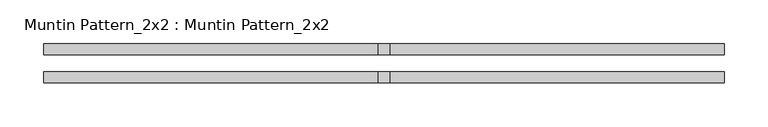
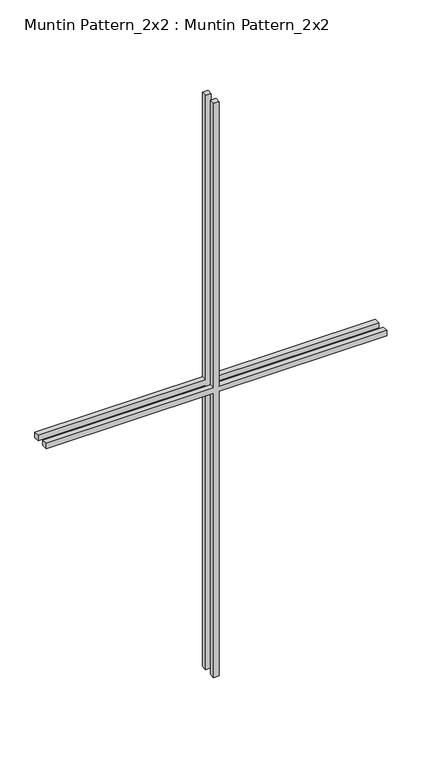
"""IFC4 building model written with IfcOpenShell, lengths in millimetres: proxy geometry, Muntin Pattern_2x2 : Muntin Pattern_2x2."""

from ifc_helpers import new_model, si_unit, frame, origin, place, context, project, spatial, polyline, outline, extrude, source, transform, mapped, element, save


def muntin_pattern_2x2_muntin_pattern_2x2_9cc8fee8(model_context):
    return source(origin(), model_context, "Body", "SweptSolid", [
        extrude(outline(polyline([(698.5, -6.35), (698.5, -388.9375), (685.8, -388.9375), (685.8, -6.35), (0.0, -6.35), (0.0, 6.35), (685.8, 6.35), (685.8, 388.9375), (698.5, 388.9375), (698.5, 6.35), (1384.3, 6.35), (1384.3, -6.35), (698.5, -6.35)])), frame((0.0, -22.225, 0.0), z_axis=(0.0, 1.0, 0.0), x_axis=(0.0, 0.0, 1.0)), (0.0, 0.0, 1.0), 12.7),
        extrude(outline(polyline([(698.5, -6.35), (698.5, -388.9375), (685.8, -388.9375), (685.8, -6.35), (0.0, -6.35), (0.0, 6.35), (685.8, 6.35), (685.8, 388.9375), (698.5, 388.9375), (698.5, 6.35), (1384.3, 6.35), (1384.3, -6.35), (698.5, -6.35)])), frame((0.0, 9.525, 0.0), z_axis=(0.0, 1.0, 0.0), x_axis=(0.0, 0.0, 1.0)), (0.0, 0.0, 1.0), 12.7),
    ])


if __name__ == "__main__":
    model = new_model("IFC4")
    model_context = context("Model", 3, world=origin())
    ifc_project = project(units=[si_unit("LENGTHUNIT", "METRE", prefix="MILLI")], contexts=[model_context])
    site = spatial("IfcSite", under=ifc_project)
    building = spatial("IfcBuilding", under=site)
    placement = place(None, origin())
    muntin_pattern_2x2_muntin_pattern_2x2_shape = muntin_pattern_2x2_muntin_pattern_2x2_9cc8fee8(model_context)
    element("IfcBuildingElementProxy", 1, Name="Muntin Pattern_2x2 : Muntin Pattern_2x2", ObjectType="Muntin Pattern_2x2 : Muntin Pattern_2x2", at=placement, inside=building, context=model_context, shape_type="MappedRepresentation", body=[
        mapped(muntin_pattern_2x2_muntin_pattern_2x2_shape, transform((0.0, 0.0, 0.0), x_axis=(1.0, 0.0, 0.0), y_axis=(0.0, 1.0, 0.0), z_axis=(0.0, 0.0, 1.0))),
    ])
    save(model, "model.ifc")

# Revit data of these elements
# Type "Muntin Pattern_2x2 : Muntin Pattern_2x2"
#   Width [instance default] = 4' - 0"
#   Thickness = 0' - 0 1/2"
#   Height [instance default] = 4' - 0"
#   Distance = 0' - 0 3/4"
#   Interior Material [instance default] = none
#   Exterior Material [instance default] = none
#   Default Elevation = 0
# Element 1 (IfcBuildingElementProxy, "Muntin Pattern_2x2 : Muntin Pattern_2x2")
#   Width = 2' - 6 5/8"
#   Height = 4' - 6 1/2"
#   Interior Material = Wood - Stained
#   Exterior Material = Clad - White
#   Materials on its faces: "Clad - White", "Wood - Stained"
# Materials
#   "Clad - White": class "Wood", colour RGB 242 242 238, transparency 0, Cost = 0
#   "Wood - Stained": class "Wood", colour RGB 224 178 126, transparency 0, Cost = 0
